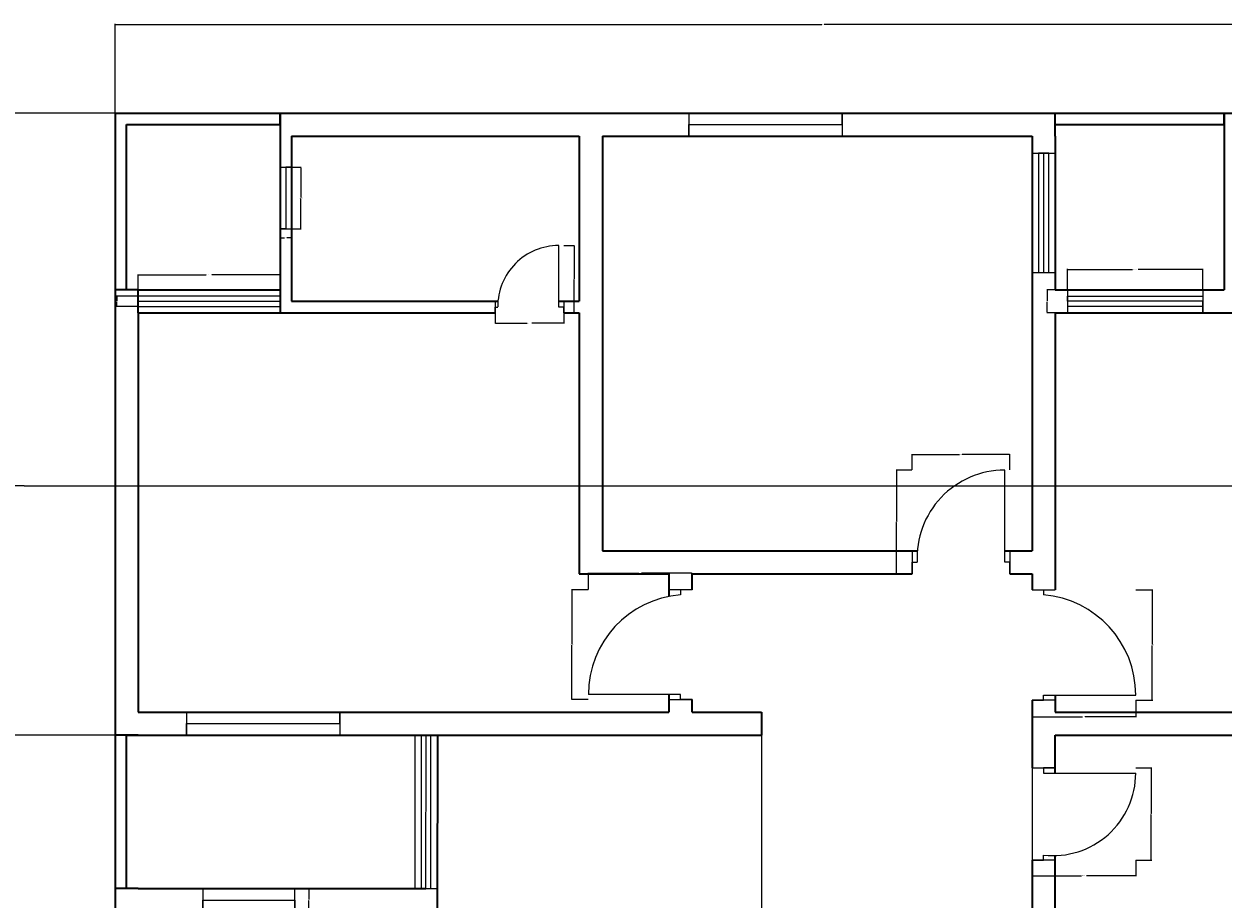
# Model space of a CAD drawing. Units: inches. Extents: x 2014 to 3678, y 870 to 2323.
# Tile 5 of 7: x 2813 to 3282, y 1376 to 1718. Entities that reach past the tile are written whole.
import ezdxf

# ---------------------------------------------------------------- set-up
doc = ezdxf.new("R2010")
doc.units = ezdxf.units.IN
for name, color, linetype, lineweight in [('A-ANNO-DIMS', 2, 'Continuous', 18), ('A-ANNO-SYMB', 2, 'Continuous', 18), ('A-DOOR', 3, 'Continuous', 18), ('A-GLAZ', 4, 'Continuous', 18), ('A-WALL', 7, 'Continuous', 35)]:
    doc.layers.add(name, color=color, linetype=linetype, lineweight=lineweight)
doc.styles.get("Standard").update_dxf_attribs({"font": 'arial.ttf'})
doc.dimstyles.get("Standard").update_dxf_attribs({"dimtxt": 0.18, "dimasz": 0.18, "dimexe": 0.18, "dimexo": 0.0625, "dimgap": 0.09, "dimtad": 0, "dimtih": 1, "dimtoh": 1, "dimdec": 4, "dimzin": 0, "dimdsep": 46, "dimtxsty": 'Standard', "dimcen": 0.09, "dimadec": 0, "dimazin": 0, "dimtfac": 1, "dimtdec": 4, "dimtofl": 0, "dimtmove": 0, "dimatfit": 3, "dimfxl": 1, "dimtolj": 1, "dimtzin": 0, "dimarcsym": 0})

# ---------------------------------------------------------------- blocks, each defined once
blk = doc.blocks.new('DOOR-BATH-WEST-24')
for p, q in [((24.83, 2.25), (24.83, 26.25)), ((0, 4.5), (0, 0)), ((0, 0), (0, 2.25)), ((0, 2.25), (1, 2.25)), ((26.83, 2.25), (24.83, 2.25)), ((26.83, 4.5), (26.83, 0)), ((26.83, 0), (26.83, 2.25))]:
    blk.add_line(p, q)
blk.add_arc((24.83, 2.42), 23.83, 90, 180.4)
blk = doc.blocks.new('DOOR-BED-CENTRE-36')
for p, q in [((36.22, 28.5), (36.22, 40.5)), ((36.22, 4.5), (36.22, 28.5)), ((0, 9), (0, 0)), ((38.22, 9), (38.22, 0)), ((0, 0), (0, 4.5)), ((0, 4.5), (2, 4.5)), ((38.22, 4.5), (36.22, 4.5)), ((38.22, 0), (38.22, 4.5))]:
    blk.add_line(p, q)
blk.add_arc((36.22, 6.23), 34.27, 90, 182.898)
blk = doc.blocks.new('DOOR-BED-WEST-36')
for p, q in [((40.5, 42.9), (31.5, 42.9)), ((36, 42.9), (36, 40.9)), ((36, 2), (0, 2)), ((36, 0), (36, 2)), ((31.5, 0), (40.5, 0)), ((40.5, 0), (36, 0))]:
    blk.add_line(p, q)
blk.add_arc((39.02, 2), 39.02, 94.441, 180)
blk = doc.blocks.new('DOOR-BED-NE-36')
for p, q in [((0, 43.13), (9, 43.13)), ((4.5, 43.13), (4.5, 41.13)), ((9, 0), (0, 0)), ((0, 0), (4.5, 0)), ((4.5, 0), (4.5, 2)), ((4.5, 2), (40.5, 2))]:
    blk.add_line(p, q)
blk.add_arc((1.23, 2), 39.27, 0, 85.2291)
blk = doc.blocks.new('DOOR-BED-SE-36')
for p, q in [((0, 36.03), (9, 36.03)), ((9, 36.03), (4.5, 36.03)), ((4.5, 36.03), (4.5, 34.03)), ((4.5, 34.03), (40.5, 34.03)), ((9, 0), (0, 0)), ((0, 0), (4.5, 0)), ((4.5, 0), (4.5, 2))]:
    blk.add_line(p, q)
blk.add_arc((8.25, 34.03), 32.25, 263.3141, 0)
blk = doc.blocks.new('WIN-60')
for p, q in [((0, 9), (0, 0)), ((60, 4.5), (60, 9)), ((60, 9), (60, 0)), ((0, 0), (0, 4.5)), ((0, 4.5), (60, 4.5))]:
    blk.add_line(p, q)
blk = doc.blocks.new('VENT-24')
for p, q in [((0, 24), (4.5, 24)), ((4.5, 24), (2.25, 24)), ((2.25, 24), (2.25, 0)), ((2.25, 0), (0, 0)), ((0, 0), (4.5, 0))]:
    blk.add_line(p, q)
blk = doc.blocks.new('WIN-36')
for p, q in [((0, 9), (0, 0)), ((36, 0), (36, 9)), ((0, 0), (0, 4.5)), ((0, 4.5), (36, 4.5)), ((36, 4.5), (36, 0))]:
    blk.add_line(p, q)
blk = doc.blocks.new('GLAZ-OTS-EAST')
for p, q in [((0, 9), (0, 0)), ((0, 5.5), (0, 6.5)), ((0, 6.5), (52.91, 6.5)), ((0, 4.5), (0, 5.5)), ((52.91, 9), (52.91, 0)), ((52.91, 6.5), (52.91, 4.5)), ((52.91, 4.5), (0, 4.5)), ((52.91, 2.5), (0, 2.5)), ((52.91, 0), (52.91, 4.5)), ((52.91, 4.5), (52.91, 2.5))]:
    blk.add_line(p, q)
blk = doc.blocks.new('GLAZ-OTS-SIDE')
for p, q in [((0, 46.57), (9, 46.57)), ((4.5, 46.57), (2.5, 46.57)), ((2.5, 46.57), (2.5, 0)), ((4.5, 46.57), (4.5, 0)), ((6.5, 46.57), (4.5, 46.57)), ((6.5, 0), (6.5, 46.57)), ((0, 0), (9, 0)), ((4.5, 0), (6.5, 0))]:
    blk.add_line(p, q)
blk = doc.blocks.new('GLAZ-OTS-WEST')
for p, q in [((55.5, 4), (0, 4)), ((0, 4), (0, 2)), ((0, 2), (55.5, 2)), ((0, 2), (0, 0)), ((0, 0), (55.5, 0)), ((55.5, 2), (55.5, 4))]:
    blk.add_line(p, q)
blk = doc.blocks.new('GLAZ-LAUNDRY')
for p, q in [((9, 60), (0, 60)), ((0, 60), (0, 0)), ((4.5, 60), (2.5, 60)), ((2.5, 60), (2.5, 0)), ((4.35, 0), (4.5, 60)), ((6.35, 0), (6.35, 60)), ((8, 60), (7, 60)), ((9, 60), (8, 60)), ((0, 0), (4.35, 0)), ((2.5, 0), (4.35, 0)), ((4.35, 0), (9, 0.03)), ((7.27, 0.02), (9, 0.03)), ((4.35, 0), (6.35, 0))]:
    blk.add_line(p, q)
blk = doc.blocks.new('*D32')
at = {"layer": 'A-ANNO-DIMS', "color": 0, "lineweight": -2, "transparency": 16777216}
for p, q in [((2917.73, 1662.02), (2921.45, 1662.02)), ((2921.27, 1661.84), (2921.27, 1650.2)), ((2921.27, 1638.2), (2921.27, 1649.84)), ((2917.73, 1638.02), (2921.45, 1638.02))]:
    blk.add_line(p, q, dxfattribs=at)
at = {"layer": 'A-ANNO-DIMS', "color": 0, "transparency": 16777216}
for points in [[(2921.24, 1661.84), (2921.3, 1661.84), (2921.27, 1662.02)], [(2921.24, 1638.2), (2921.3, 1638.2), (2921.27, 1638.02)]]:
    blk.add_solid(points, dxfattribs=at)
at = {"layer": 'Defpoints', "color": 0, "transparency": 16777216}
for p in [(2917.67, 1662.02), (2921.27, 1662.02), (2917.67, 1638.02)]:
    blk.add_point(p, dxfattribs=at)
at = {"layer": 'A-ANNO-DIMS', "color": 0, "transparency": 16777216, "insert": (2921.27, 1650.02), "char_height": 0.18, "attachment_point": 5}
blk.add_mtext('\\A1;VENT 24 TYP.', dxfattribs=at)
blk = doc.blocks.new('*D33')
at = {"layer": 'A-ANNO-DIMS', "color": 0, "lineweight": -2, "transparency": 16777216}
for p, q in [((2913.17, 1637.95), (2913.17, 1634.24)), ((2917.67, 1637.95), (2917.67, 1634.24)), ((2913.35, 1634.42), (2914.96, 1634.42)), ((2917.49, 1634.42), (2915.88, 1634.42))]:
    blk.add_line(p, q, dxfattribs=at)
at = {"layer": 'A-ANNO-DIMS', "color": 0, "transparency": 16777216}
for points in [[(2913.35, 1634.45), (2913.35, 1634.39), (2913.17, 1634.42)], [(2917.49, 1634.45), (2917.49, 1634.39), (2917.67, 1634.42)]]:
    blk.add_solid(points, dxfattribs=at)
at = {"layer": 'Defpoints', "color": 0, "transparency": 16777216}
for p in [(2913.17, 1638.02), (2917.67, 1638.02), (2917.67, 1634.42)]:
    blk.add_point(p, dxfattribs=at)
at = {"layer": 'A-ANNO-DIMS', "color": 0, "transparency": 16777216, "insert": (2915.42, 1634.42), "char_height": 0.18, "attachment_point": 5}
blk.add_mtext('\\A1;5 TYP.', dxfattribs=at)
blk = doc.blocks.new('*D36')
at = {"layer": 'A-ANNO-DIMS', "color": 0, "lineweight": -2, "transparency": 16777216}
for p, q in [((2997.28, 1605.1), (2997.28, 1600.96)), ((3024.11, 1605.1), (3024.11, 1600.96)), ((2997.46, 1601.14), (3009.76, 1601.14)), ((3023.93, 1601.14), (3011.63, 1601.14))]:
    blk.add_line(p, q, dxfattribs=at)
at = {"layer": 'A-ANNO-DIMS', "color": 0, "transparency": 16777216}
for points in [[(2997.46, 1601.17), (2997.46, 1601.11), (2997.28, 1601.14)], [(3023.93, 1601.17), (3023.93, 1601.11), (3024.11, 1601.14)]]:
    blk.add_solid(points, dxfattribs=at)
at = {"layer": 'Defpoints', "color": 0, "transparency": 16777216}
for p in [(2997.28, 1605.17), (3024.11, 1605.17), (3024.11, 1601.14)]:
    blk.add_point(p, dxfattribs=at)
at = {"layer": 'A-ANNO-DIMS', "color": 0, "transparency": 16777216, "insert": (3010.69, 1601.14), "char_height": 0.18, "attachment_point": 5}
blk.add_mtext('\\A1;DOOR 27 TYP.', dxfattribs=at)
blk = doc.blocks.new('*D37')
at = {"layer": 'A-ANNO-DIMS', "color": 0, "lineweight": -2, "transparency": 16777216}
for p, q in [((3024.17, 1631.42), (3028.31, 1631.42)), ((3028.13, 1631.24), (3028.13, 1618.47)), ((3028.13, 1605.35), (3028.13, 1618.11)), ((3024.17, 1605.17), (3028.31, 1605.17))]:
    blk.add_line(p, q, dxfattribs=at)
at = {"layer": 'A-ANNO-DIMS', "color": 0, "transparency": 16777216}
for points in [[(3028.1, 1631.24), (3028.16, 1631.24), (3028.13, 1631.42)], [(3028.1, 1605.35), (3028.16, 1605.35), (3028.13, 1605.17)]]:
    blk.add_solid(points, dxfattribs=at)
at = {"layer": 'Defpoints', "color": 0, "transparency": 16777216}
for p in [(3024.11, 1631.42), (3028.13, 1631.42), (3024.11, 1605.17)]:
    blk.add_point(p, dxfattribs=at)
at = {"layer": 'A-ANNO-DIMS', "color": 0, "transparency": 16777216, "insert": (3028.13, 1618.29), "char_height": 0.18, "attachment_point": 5}
blk.add_mtext('\\A1;26 TYP.', dxfattribs=at)
blk = doc.blocks.new('*D38')
at = {"layer": 'A-ANNO-DIMS', "color": 0, "lineweight": -2, "transparency": 16777216}
for p, q in [((3160.16, 1543.67), (3153.97, 1543.67)), ((3154.15, 1543.49), (3154.15, 1523.6)), ((3154.15, 1503.35), (3154.15, 1523.23)), ((3160.16, 1503.17), (3153.97, 1503.17))]:
    blk.add_line(p, q, dxfattribs=at)
at = {"layer": 'A-ANNO-DIMS', "color": 0, "transparency": 16777216}
for points in [[(3154.12, 1543.49), (3154.18, 1543.49), (3154.15, 1543.67)], [(3154.12, 1503.35), (3154.18, 1503.35), (3154.15, 1503.17)]]:
    blk.add_solid(points, dxfattribs=at)
at = {"layer": 'Defpoints', "color": 0, "transparency": 16777216}
for p in [(3154.15, 1543.67), (3160.23, 1543.67), (3160.23, 1503.17)]:
    blk.add_point(p, dxfattribs=at)
at = {"layer": 'A-ANNO-DIMS', "color": 0, "transparency": 16777216, "insert": (3154.15, 1523.42), "char_height": 0.18, "attachment_point": 5}
blk.add_mtext('\\A1;DOOR 41 TYP.', dxfattribs=at)
blk = doc.blocks.new('*D39')
at = {"layer": 'A-ANNO-DIMS', "color": 0, "lineweight": -2, "transparency": 16777216}
for p, q in [((3160.23, 1543.73), (3160.23, 1549.92)), ((3160.41, 1549.74), (3178.81, 1549.74)), ((3198.27, 1549.74), (3179.87, 1549.74)), ((3198.45, 1543.73), (3198.45, 1549.92))]:
    blk.add_line(p, q, dxfattribs=at)
at = {"layer": 'A-ANNO-DIMS', "color": 0, "transparency": 16777216}
for points in [[(3160.41, 1549.77), (3160.41, 1549.71), (3160.23, 1549.74)], [(3198.27, 1549.77), (3198.27, 1549.71), (3198.45, 1549.74)]]:
    blk.add_solid(points, dxfattribs=at)
at = {"layer": 'Defpoints', "color": 0, "transparency": 16777216}
for p in [(3198.45, 1549.74), (3160.23, 1543.67), (3198.45, 1543.67)]:
    blk.add_point(p, dxfattribs=at)
at = {"layer": 'A-ANNO-DIMS', "color": 0, "transparency": 16777216, "insert": (3179.34, 1549.74), "char_height": 0.18, "attachment_point": 5}
blk.add_mtext('\\A1;38 TYP.', dxfattribs=at)
blk = doc.blocks.new('*D40')
at = {"layer": 'A-ANNO-DIMS', "color": 0, "lineweight": -2, "transparency": 16777216}
for p, q in [((3033.65, 1496.94), (3027.1, 1496.94)), ((3027.28, 1496.76), (3027.28, 1475.67)), ((3027.28, 1454.21), (3027.28, 1475.3)), ((3033.65, 1454.03), (3027.1, 1454.03))]:
    blk.add_line(p, q, dxfattribs=at)
at = {"layer": 'A-ANNO-DIMS', "color": 0, "transparency": 16777216}
for points in [[(3027.25, 1496.76), (3027.31, 1496.76), (3027.28, 1496.94)], [(3027.25, 1454.21), (3027.31, 1454.21), (3027.28, 1454.03)]]:
    blk.add_solid(points, dxfattribs=at)
at = {"layer": 'Defpoints', "color": 0, "transparency": 16777216}
for p in [(3027.28, 1496.94), (3033.71, 1496.94), (3033.71, 1454.03)]:
    blk.add_point(p, dxfattribs=at)
at = {"layer": 'A-ANNO-DIMS', "color": 0, "transparency": 16777216, "insert": (3027.28, 1475.49), "char_height": 0.18, "attachment_point": 5}
blk.add_mtext('\\A1;DOOR 43 TYP.', dxfattribs=at)
blk = doc.blocks.new('*D41')
at = {"layer": 'A-ANNO-DIMS', "color": 0, "lineweight": -2, "transparency": 16777216}
for p, q in [((3033.71, 1497), (3033.71, 1503.55)), ((3033.89, 1503.37), (3053.43, 1503.37)), ((3074.03, 1503.37), (3054.5, 1503.37)), ((3074.21, 1497), (3074.21, 1503.55))]:
    blk.add_line(p, q, dxfattribs=at)
at = {"layer": 'A-ANNO-DIMS', "color": 0, "transparency": 16777216}
for points in [[(3033.89, 1503.4), (3033.89, 1503.34), (3033.71, 1503.37)], [(3074.03, 1503.4), (3074.03, 1503.34), (3074.21, 1503.37)]]:
    blk.add_solid(points, dxfattribs=at)
at = {"layer": 'Defpoints', "color": 0, "transparency": 16777216}
for p in [(3074.21, 1503.37), (3033.71, 1496.94), (3074.21, 1496.94)]:
    blk.add_point(p, dxfattribs=at)
at = {"layer": 'A-ANNO-DIMS', "color": 0, "transparency": 16777216, "insert": (3053.96, 1503.37), "char_height": 0.18, "attachment_point": 5}
blk.add_mtext('\\A1;41 TYP.', dxfattribs=at)
blk = doc.blocks.new('*D42')
at = {"layer": 'A-ANNO-DIMS', "color": 0, "lineweight": -2, "transparency": 16777216}
for p, q in [((3247.73, 1496.94), (3254.32, 1496.94)), ((3254.14, 1496.76), (3254.14, 1475.56)), ((3254.14, 1453.99), (3254.14, 1475.19)), ((3247.73, 1453.81), (3254.32, 1453.81))]:
    blk.add_line(p, q, dxfattribs=at)
at = {"layer": 'A-ANNO-DIMS', "color": 0, "transparency": 16777216}
for points in [[(3254.11, 1496.76), (3254.17, 1496.76), (3254.14, 1496.94)], [(3254.11, 1453.99), (3254.17, 1453.99), (3254.14, 1453.81)]]:
    blk.add_solid(points, dxfattribs=at)
at = {"layer": 'Defpoints', "color": 0, "transparency": 16777216}
for p in [(3247.67, 1496.94), (3254.14, 1496.94), (3247.67, 1453.81)]:
    blk.add_point(p, dxfattribs=at)
at = {"layer": 'A-ANNO-DIMS', "color": 0, "transparency": 16777216, "insert": (3254.14, 1475.37), "char_height": 0.18, "attachment_point": 5}
blk.add_mtext('\\A1;DOOR 43 TYP.', dxfattribs=at)
blk = doc.blocks.new('*D43')
at = {"layer": 'A-ANNO-DIMS', "color": 0, "lineweight": -2, "transparency": 16777216}
for p, q in [((3207.17, 1453.75), (3207.17, 1447.16)), ((3247.67, 1453.75), (3247.67, 1447.16)), ((3207.35, 1447.34), (3226.89, 1447.34)), ((3247.49, 1447.34), (3227.95, 1447.34))]:
    blk.add_line(p, q, dxfattribs=at)
at = {"layer": 'A-ANNO-DIMS', "color": 0, "transparency": 16777216}
for points in [[(3207.35, 1447.37), (3207.35, 1447.31), (3207.17, 1447.34)], [(3247.49, 1447.37), (3247.49, 1447.31), (3247.67, 1447.34)]]:
    blk.add_solid(points, dxfattribs=at)
at = {"layer": 'Defpoints', "color": 0, "transparency": 16777216}
for p in [(3207.17, 1453.81), (3247.67, 1453.81), (3247.67, 1447.34)]:
    blk.add_point(p, dxfattribs=at)
at = {"layer": 'A-ANNO-DIMS', "color": 0, "transparency": 16777216, "insert": (3227.42, 1447.34), "char_height": 0.18, "attachment_point": 5}
blk.add_mtext('\\A1;41 TYP.', dxfattribs=at)
blk = doc.blocks.new('*D44')
at = {"layer": 'A-ANNO-DIMS', "color": 0, "lineweight": -2, "transparency": 16777216}
for p, q in [((3207.17, 1391.22), (3207.17, 1385.03)), ((3247.67, 1391.22), (3247.67, 1385.03)), ((3207.35, 1385.21), (3226.49, 1385.21)), ((3247.49, 1385.21), (3228.36, 1385.21))]:
    blk.add_line(p, q, dxfattribs=at)
at = {"layer": 'A-ANNO-DIMS', "color": 0, "transparency": 16777216}
for points in [[(3207.35, 1385.24), (3207.35, 1385.18), (3207.17, 1385.21)], [(3247.49, 1385.24), (3247.49, 1385.18), (3247.67, 1385.21)]]:
    blk.add_solid(points, dxfattribs=at)
at = {"layer": 'Defpoints', "color": 0, "transparency": 16777216}
for p in [(3207.17, 1391.28), (3247.67, 1391.28), (3247.67, 1385.21)]:
    blk.add_point(p, dxfattribs=at)
at = {"layer": 'A-ANNO-DIMS', "color": 0, "transparency": 16777216, "insert": (3227.42, 1385.21), "char_height": 0.18, "attachment_point": 5}
blk.add_mtext('\\A1;DOOR 41 TYP.', dxfattribs=at)
blk = doc.blocks.new('*D45')
at = {"layer": 'A-ANNO-DIMS', "color": 0, "lineweight": -2, "transparency": 16777216}
for p, q in [((3247.73, 1427.31), (3253.93, 1427.31)), ((3253.75, 1427.13), (3253.75, 1409.48)), ((3253.75, 1391.46), (3253.75, 1409.11)), ((3247.73, 1391.28), (3253.93, 1391.28))]:
    blk.add_line(p, q, dxfattribs=at)
at = {"layer": 'A-ANNO-DIMS', "color": 0, "transparency": 16777216}
for points in [[(3253.72, 1427.13), (3253.78, 1427.13), (3253.75, 1427.31)], [(3253.72, 1391.46), (3253.78, 1391.46), (3253.75, 1391.28)]]:
    blk.add_solid(points, dxfattribs=at)
at = {"layer": 'Defpoints', "color": 0, "transparency": 16777216}
for p in [(3247.67, 1427.31), (3253.75, 1427.31), (3247.67, 1391.28)]:
    blk.add_point(p, dxfattribs=at)
at = {"layer": 'A-ANNO-DIMS', "color": 0, "transparency": 16777216, "insert": (3253.75, 1409.29), "char_height": 0.18, "attachment_point": 5}
blk.add_mtext('\\A1;36 TYP.', dxfattribs=at)
blk = doc.blocks.new('*D55')
at = {"layer": 'A-ANNO-DIMS', "color": 0, "lineweight": -2, "transparency": 16777216}
for p, q in [((2919.09, 1380.17), (2924.6, 1380.17)), ((2924.42, 1379.99), (2924.42, 1375.85)), ((2924.42, 1371.35), (2924.42, 1375.48)), ((2919.09, 1371.17), (2924.6, 1371.17))]:
    blk.add_line(p, q, dxfattribs=at)
at = {"layer": 'A-ANNO-DIMS', "color": 0, "transparency": 16777216}
for points in [[(2924.39, 1379.99), (2924.45, 1379.99), (2924.42, 1380.17)], [(2924.39, 1371.35), (2924.45, 1371.35), (2924.42, 1371.17)]]:
    blk.add_solid(points, dxfattribs=at)
at = {"layer": 'Defpoints', "color": 0, "transparency": 16777216}
for p in [(2919.02, 1380.17), (2924.42, 1380.17), (2919.02, 1371.17)]:
    blk.add_point(p, dxfattribs=at)
at = {"layer": 'A-ANNO-DIMS', "color": 0, "transparency": 16777216, "insert": (2924.42, 1375.67), "char_height": 0.18, "attachment_point": 5}
blk.add_mtext('\\A1;9 TYP.', dxfattribs=at)
blk = doc.blocks.new('*D56')
at = {"layer": 'A-ANNO-DIMS', "color": 0, "lineweight": -2, "transparency": 16777216}
for p, q in [((3221.02, 1614.23), (3221.02, 1622.28)), ((3221.2, 1622.1), (3246.36, 1622.1)), ((3273.75, 1622.1), (3248.59, 1622.1)), ((3273.93, 1614.23), (3273.93, 1622.28))]:
    blk.add_line(p, q, dxfattribs=at)
at = {"layer": 'A-ANNO-DIMS', "color": 0, "transparency": 16777216}
for points in [[(3221.2, 1622.13), (3221.2, 1622.07), (3221.02, 1622.1)], [(3273.75, 1622.13), (3273.75, 1622.07), (3273.93, 1622.1)]]:
    blk.add_solid(points, dxfattribs=at)
at = {"layer": 'Defpoints', "color": 0, "transparency": 16777216}
for p in [(3273.93, 1622.1), (3221.02, 1614.17), (3273.93, 1614.17)]:
    blk.add_point(p, dxfattribs=at)
at = {"layer": 'A-ANNO-DIMS', "color": 0, "transparency": 16777216, "insert": (3247.48, 1622.1), "char_height": 0.18, "attachment_point": 5}
blk.add_mtext('\\A1;GLAZING 53 TYP.', dxfattribs=at)
blk = doc.blocks.new('*D57')
at = {"layer": 'A-ANNO-DIMS', "color": 0, "lineweight": -2, "transparency": 16777216}
for p, q in [((3220.96, 1614.17), (3212.91, 1614.17)), ((3213.09, 1613.99), (3213.09, 1609.85)), ((3213.09, 1605.35), (3213.09, 1609.48)), ((3220.96, 1605.17), (3212.91, 1605.17))]:
    blk.add_line(p, q, dxfattribs=at)
at = {"layer": 'A-ANNO-DIMS', "color": 0, "transparency": 16777216}
for points in [[(3213.06, 1613.99), (3213.12, 1613.99), (3213.09, 1614.17)], [(3213.06, 1605.35), (3213.12, 1605.35), (3213.09, 1605.17)]]:
    blk.add_solid(points, dxfattribs=at)
at = {"layer": 'Defpoints', "color": 0, "transparency": 16777216}
for p in [(3213.09, 1614.17), (3221.02, 1614.17), (3221.02, 1605.17)]:
    blk.add_point(p, dxfattribs=at)
at = {"layer": 'A-ANNO-DIMS', "color": 0, "transparency": 16777216, "insert": (3213.09, 1609.67), "char_height": 0.18, "attachment_point": 5}
blk.add_mtext('\\A1;9 TYP.', dxfattribs=at)
blk = doc.blocks.new('*D60')
at = {"layer": 'A-ANNO-DIMS', "color": 0, "lineweight": -2, "transparency": 16777216}
for p, q in [((2857.67, 1611.73), (2857.67, 1620.17)), ((2857.85, 1619.99), (2884.31, 1619.99)), ((2912.99, 1619.99), (2886.54, 1619.99)), ((2913.17, 1611.73), (2913.17, 1620.17))]:
    blk.add_line(p, q, dxfattribs=at)
at = {"layer": 'A-ANNO-DIMS', "color": 0, "transparency": 16777216}
for points in [[(2857.85, 1620.02), (2857.85, 1619.96), (2857.67, 1619.99)], [(2912.99, 1620.02), (2912.99, 1619.96), (2913.17, 1619.99)]]:
    blk.add_solid(points, dxfattribs=at)
at = {"layer": 'Defpoints', "color": 0, "transparency": 16777216}
for p in [(2913.17, 1619.99), (2857.67, 1611.67), (2913.17, 1611.67)]:
    blk.add_point(p, dxfattribs=at)
at = {"layer": 'A-ANNO-DIMS', "color": 0, "transparency": 16777216, "insert": (2885.42, 1619.99), "char_height": 0.18, "attachment_point": 5}
blk.add_mtext('\\A1;GLAZING 56 TYP.', dxfattribs=at)
blk = doc.blocks.new('*D61')
at = {"layer": 'A-ANNO-DIMS', "color": 0, "lineweight": -2, "transparency": 16777216}
for p, q in [((2857.61, 1611.67), (2849.17, 1611.67)), ((2849.35, 1611.49), (2849.35, 1609.85)), ((2849.35, 1607.85), (2849.35, 1609.49)), ((2857.61, 1607.67), (2849.17, 1607.67))]:
    blk.add_line(p, q, dxfattribs=at)
at = {"layer": 'A-ANNO-DIMS', "color": 0, "transparency": 16777216}
for points in [[(2849.32, 1611.49), (2849.38, 1611.49), (2849.35, 1611.67)], [(2849.32, 1607.85), (2849.38, 1607.85), (2849.35, 1607.67)]]:
    blk.add_solid(points, dxfattribs=at)
at = {"layer": 'Defpoints', "color": 0, "transparency": 16777216}
for p in [(2849.35, 1611.67), (2857.67, 1611.67), (2857.67, 1607.67)]:
    blk.add_point(p, dxfattribs=at)
at = {"layer": 'A-ANNO-DIMS', "color": 0, "transparency": 16777216, "insert": (2849.35, 1609.67), "char_height": 0.18, "attachment_point": 5}
blk.add_mtext('\\A1;4 TYP.', dxfattribs=at)
blk = doc.blocks.new('*D91')
at = {"layer": 'A-ANNO-DIMS', "color": 0, "lineweight": -2, "transparency": 16777216}
for p, q in [((2848.67, 1683.23), (2848.67, 1718)), ((2848.85, 1717.82), (3125.03, 1717.82)), ((3401.99, 1717.82), (3125.82, 1717.82)), ((3402.17, 1683.23), (3402.17, 1718))]:
    blk.add_line(p, q, dxfattribs=at)
at = {"layer": 'A-ANNO-DIMS', "color": 0, "transparency": 16777216}
for points in [[(2848.85, 1717.85), (2848.85, 1717.79), (2848.67, 1717.82)], [(3401.99, 1717.85), (3401.99, 1717.79), (3402.17, 1717.82)]]:
    blk.add_solid(points, dxfattribs=at)
at = {"layer": 'Defpoints', "color": 0, "transparency": 16777216}
for p in [(3402.17, 1717.82), (2848.67, 1683.17), (3402.17, 1683.17)]:
    blk.add_point(p, dxfattribs=at)
at = {"layer": 'A-ANNO-DIMS', "color": 0, "transparency": 16777216, "insert": (3125.42, 1717.82), "char_height": 0.18, "attachment_point": 5}
blk.add_mtext('\\A1;553.5', dxfattribs=at)
blk = doc.blocks.new('*D95')
at = {"layer": 'A-ANNO-DIMS', "color": 0, "lineweight": -2, "transparency": 16777216}
for p, q in [((2848.61, 1440.17), (2778.34, 1440.17)), ((2778.52, 1439.99), (2778.52, 1405.85)), ((2778.52, 1371.35), (2778.52, 1405.48)), ((2857.61, 1371.17), (2778.34, 1371.17))]:
    blk.add_line(p, q, dxfattribs=at)
at = {"layer": 'A-ANNO-DIMS', "color": 0, "transparency": 16777216}
for points in [[(2778.49, 1439.99), (2778.55, 1439.99), (2778.52, 1440.17)], [(2778.49, 1371.35), (2778.55, 1371.35), (2778.52, 1371.17)]]:
    blk.add_solid(points, dxfattribs=at)
at = {"layer": 'Defpoints', "color": 0, "transparency": 16777216}
for p in [(2778.52, 1440.17), (2848.67, 1440.17), (2857.67, 1371.17)]:
    blk.add_point(p, dxfattribs=at)
at = {"layer": 'A-ANNO-DIMS', "color": 0, "transparency": 16777216, "insert": (2778.52, 1405.67), "char_height": 0.18, "attachment_point": 5}
blk.add_mtext('\\A1;69', dxfattribs=at)
blk = doc.blocks.new('*D96')
at = {"layer": 'A-ANNO-DIMS', "color": 0, "lineweight": -2, "transparency": 16777216}
for p, q in [((2813.11, 1537.5), (2778.34, 1537.5)), ((2778.52, 1537.32), (2778.52, 1489.01)), ((2778.52, 1440.35), (2778.52, 1488.65)), ((2848.61, 1440.17), (2778.34, 1440.17))]:
    blk.add_line(p, q, dxfattribs=at)
at = {"layer": 'A-ANNO-DIMS', "color": 0, "transparency": 16777216}
for points in [[(2778.49, 1537.32), (2778.55, 1537.32), (2778.52, 1537.5)], [(2778.49, 1440.35), (2778.55, 1440.35), (2778.52, 1440.17)]]:
    blk.add_solid(points, dxfattribs=at)
at = {"layer": 'Defpoints', "color": 0, "transparency": 16777216}
for p in [(2778.52, 1537.5), (2813.17, 1537.5), (2848.67, 1440.17)]:
    blk.add_point(p, dxfattribs=at)
at = {"layer": 'A-ANNO-DIMS', "color": 0, "transparency": 16777216, "insert": (2778.52, 1488.83), "char_height": 0.18, "attachment_point": 5}
blk.add_mtext('\\A1;97.33', dxfattribs=at)
blk = doc.blocks.new('*D97')
at = {"layer": 'A-ANNO-DIMS', "color": 0, "lineweight": -2, "transparency": 16777216}
for p, q in [((2848.61, 1683.17), (2778.34, 1683.17)), ((2778.52, 1682.99), (2778.52, 1610.51)), ((2778.52, 1537.68), (2778.52, 1610.15)), ((2813.11, 1537.5), (2778.34, 1537.5))]:
    blk.add_line(p, q, dxfattribs=at)
at = {"layer": 'A-ANNO-DIMS', "color": 0, "transparency": 16777216}
for points in [[(2778.49, 1682.99), (2778.55, 1682.99), (2778.52, 1683.17)], [(2778.49, 1537.68), (2778.55, 1537.68), (2778.52, 1537.5)]]:
    blk.add_solid(points, dxfattribs=at)
at = {"layer": 'Defpoints', "color": 0, "transparency": 16777216}
for p in [(2778.52, 1683.17), (2848.67, 1683.17), (2813.17, 1537.5)]:
    blk.add_point(p, dxfattribs=at)
at = {"layer": 'A-ANNO-DIMS', "color": 0, "transparency": 16777216, "insert": (2778.52, 1610.33), "char_height": 0.18, "attachment_point": 5}
blk.add_mtext('\\A1;145.67', dxfattribs=at)
blk = doc.blocks.new('*D100')
at = {"layer": 'A-ANNO-DIMS', "color": 0, "lineweight": -2, "transparency": 16777216}
for p, q in [((3101.37, 1440.1), (3101.37, 964.34)), ((3207.17, 1427.25), (3207.17, 964.34)), ((3101.55, 964.52), (3153.88, 964.52)), ((3206.99, 964.52), (3154.65, 964.52))]:
    blk.add_line(p, q, dxfattribs=at)
at = {"layer": 'A-ANNO-DIMS', "color": 0, "transparency": 16777216}
for points in [[(3101.55, 964.55), (3101.55, 964.49), (3101.37, 964.52)], [(3206.99, 964.55), (3206.99, 964.49), (3207.17, 964.52)]]:
    blk.add_solid(points, dxfattribs=at)
at = {"layer": 'Defpoints', "color": 0, "transparency": 16777216}
for p in [(3101.37, 1440.17), (3207.17, 1427.31), (3207.17, 964.52)]:
    blk.add_point(p, dxfattribs=at)
at = {"layer": 'A-ANNO-DIMS', "color": 0, "transparency": 16777216, "insert": (3154.27, 964.52), "char_height": 0.18, "attachment_point": 5}
blk.add_mtext('\\A1;105.8', dxfattribs=at)

msp = doc.modelspace()

# ---------------------------------------------------------------- linework, layer by layer
at = {"layer": 'A-ANNO-SYMB'}
msp.add_line((2813.1731, 1537.5002), (3449.5026, 1537.5002), dxfattribs=at)
at = {"layer": 'A-WALL'}
for p, q in [((2848.6718, 1683.1655), (3402.1718, 1683.1655)), ((2848.6718, 1683.1655), (3402.1718, 1683.1655)), ((2848.6718, 1683.1655), (2848.6718, 1083.1655)), ((2913.1718, 1678.6655), (2913.1718, 1683.1655)), ((2913.1718, 1683.1655), (2913.1718, 1674.1655)), ((3216.1718, 1678.6655), (3216.1718, 1683.1655)), ((3282.1718, 1678.6655), (3282.1718, 1683.1655)), ((3282.1718, 1683.1655), (3282.1718, 1674.1655)), ((2853.1718, 1614.1655), (2853.1718, 1678.6655)), ((2853.1718, 1678.6655), (2913.1718, 1678.6655)), ((3216.1718, 1674.1655), (3216.1718, 1678.6655)), ((3216.1718, 1678.6655), (3282.1718, 1678.6655)), ((2913.1718, 1674.1655), (2913.1718, 1605.1655)), ((2917.6718, 1674.1655), (3030.1718, 1674.1655)), ((2917.6718, 1674.1655), (2917.6718, 1614.1655)), ((3030.1718, 1674.1655), (3030.1718, 1609.6655)), ((3039.1718, 1674.1655), (3207.1718, 1674.1655)), ((3039.1718, 1674.1655), (3039.1718, 1512.1655)), ((3207.1718, 1674.1655), (3207.1718, 1614.1655)), ((3216.1718, 1674.1655), (3216.1718, 1614.1655)), ((3282.1718, 1674.1655), (3282.1718, 1614.1655)), ((3207.1718, 1620.9201), (3207.1718, 1512.1655)), ((2857.6718, 1614.1655), (2848.6718, 1614.1655)), ((2857.6718, 1614.1655), (2853.1718, 1614.1655)), ((2857.6718, 1614.1655), (2913.1718, 1614.1655)), ((2857.6718, 1605.1655), (2857.6718, 1614.1655)), ((2917.6718, 1614.1655), (2917.6718, 1609.6655)), ((3216.1718, 1614.1655), (3282.1718, 1614.1655)), ((2917.6718, 1609.6655), (2998.3665, 1609.6655)), ((3022.1088, 1609.6655), (3030.1718, 1609.6655)), ((2857.6718, 1605.1655), (2997.2758, 1605.1655)), ((2857.6718, 1605.1655), (2857.6718, 1449.1655)), ((3024.1088, 1605.1655), (3030.1718, 1605.1655)), ((3030.1718, 1605.1655), (3030.1718, 1503.1655)), ((3216.1718, 1605.1655), (3360.6647, 1605.1655)), ((3216.1718, 1605.1655), (3216.1718, 1503.1655)), ((3039.1718, 1512.1655), (3162.2942, 1512.1655)), ((3196.4497, 1512.1655), (3207.1718, 1512.1655)), ((3030.1718, 1503.1655), (3065.2147, 1503.1655)), ((3065.2147, 1503.1655), (3065.2147, 1494.3233)), ((3074.2147, 1503.1655), (3160.2261, 1503.1655)), ((3074.2147, 1496.9379), (3074.2147, 1503.1655)), ((3198.4497, 1503.1655), (3207.1718, 1503.1655)), ((3207.1718, 1503.1655), (3207.1718, 1496.9379)), ((3216.1718, 1503.1655), (3216.1718, 1496.9379)), ((3065.2147, 1456.0336), (3065.2147, 1449.1655)), ((3216.1718, 1455.8082), (3216.1718, 1449.1655)), ((3074.2147, 1449.1655), (3074.2147, 1454.0336)), ((3207.1718, 1453.8082), (3207.1718, 1440.1655)), ((2857.6718, 1449.1655), (3065.2147, 1449.1655)), ((2970.1718, 1449.1655), (2979.1718, 1449.1655)), ((3074.2147, 1449.1655), (3101.3665, 1449.1655)), ((3101.3665, 1449.1655), (3101.3665, 1440.1655)), ((3216.1718, 1449.1655), (3393.1718, 1449.1655)), ((2857.6718, 1440.1655), (2848.6718, 1440.1655)), ((2853.1718, 1380.1655), (2853.1718, 1440.1655)), ((2853.1718, 1440.1655), (2857.6718, 1440.1655)), ((2857.6718, 1440.1655), (2970.1718, 1440.1655)), ((2970.1718, 1440.1655), (2979.2119, 1440.1655)), ((2974.6718, 1371.1655), (2974.8253, 1440.1655)), ((2979.2119, 1440.1655), (3101.3665, 1440.1655)), ((3207.1718, 1440.1655), (3207.1718, 1427.3075)), ((3216.1718, 1440.1655), (3393.1718, 1440.1655)), ((3216.1718, 1425.3075), (3216.1718, 1440.1655)), ((3207.1718, 1391.2811), (3207.1718, 1275.1655)), ((3216.1718, 1284.1655), (3216.1718, 1393.0704)), ((2853.1718, 1380.1655), (2848.6718, 1380.1655)), ((2857.6718, 1380.1655), (2853.1718, 1380.1655)), ((2857.6718, 1380.1655), (2970.1718, 1380.1655))]:
    msp.add_line(p, q, dxfattribs=at)

# ---------------------------------------------------------------- block references
at = {"layer": 'A-DOOR'}
for name, p in [('DOOR-BATH-WEST-24', (2997.2761, 1605.165)), ('DOOR-BED-CENTRE-36', (3160.2261, 1503.165)), ('DOOR-BED-WEST-36', (3033.7151, 1454.034)), ('DOOR-BED-NE-36', (3207.1721, 1453.808)), ('DOOR-BED-SE-36', (3207.1721, 1391.281))]:
    msp.add_blockref(name, p, dxfattribs=at)
at = {"layer": 'A-GLAZ'}
for name, p in [('WIN-60', (3072.9262, 1674.165)), ('GLAZ-OTS-SIDE', (3207.1721, 1620.92)), ('VENT-24', (2913.1721, 1638.0168)), ('GLAZ-OTS-EAST', (3221.0211, 1605.165)), ('GLAZ-OTS-WEST', (2857.6721, 1607.665)), ('WIN-60', (2876.5803, 1440.165)), ('GLAZ-LAUNDRY', (2965.8251, 1380.161)), ('WIN-36', (2883.0251, 1371.165))]:
    msp.add_blockref(name, p, dxfattribs=at)

# ---------------------------------------------------------------- dimensions: what is measured, and where the dimension line sits
at = {"layer": 'A-ANNO-DIMS'}
for base, p1, p2, picture, middle in [((3402.1718, 1717.8155), (2848.6718, 1683.1655), (3402.1718, 1683.1655), '*D91', (3125.4218, 1717.8155)), ((3207.1718, 964.5155), (3101.3665, 1440.1655), (3207.1718, 1427.3075), '*D100', (3154.2691, 964.5155))]:
    dim = msp.add_linear_dim(base=base, p1=p1, p2=p2, dimstyle='Standard', override={"dimdec": 1, "dimlfac": 1, "dimrnd": 0, "dimzin": 0, "dimdsep": 46, "dimlunit": 2}, dxfattribs=at)
    dim.commit()
    dim.dimension.update_dxf_attribs({"geometry": picture, "text_midpoint": middle})
for base, p1, p2, override, picture, middle in [((2778.5231, 1683.1655), (2813.1731, 1537.5002), (2848.6718, 1683.1655), {"dimdec": 2, "dimlfac": 1, "dimrnd": 0, "dimzin": 0, "dimdsep": 46, "dimlunit": 2}, '*D97', (2778.5231, 1610.3328)), ((2778.5231, 1537.5002), (2848.6718, 1440.1655), (2813.1731, 1537.5002), {"dimdec": 2, "dimlfac": 1, "dimrnd": 0, "dimzin": 0, "dimdsep": 46, "dimlunit": 2}, '*D96', (2778.5231, 1488.8328)), ((2778.5231, 1440.1655), (2857.6718, 1371.1655), (2848.6718, 1440.1655), {"dimdec": 0, "dimlfac": 1, "dimrnd": 0, "dimzin": 0, "dimdsep": 46, "dimlunit": 2}, '*D95', (2778.5231, 1405.6655))]:
    dim = msp.add_linear_dim(base=base, p1=p1, p2=p2, angle=90, dimstyle='Standard', override=override, dxfattribs=at)
    dim.commit()
    dim.dimension.update_dxf_attribs({"geometry": picture, "text_midpoint": middle})
for base, p1, p2, text, picture, middle in [((2921.2718, 1662.0164), (2917.6718, 1638.0164), (2917.6718, 1662.0164), 'VENT <> TYP.', '*D32', (2921.2718, 1650.0164)), ((3028.1338, 1631.4155), (3024.1088, 1605.1655), (3024.1088, 1631.4155), '<> TYP.', '*D37', (3028.1338, 1618.2905)), ((3213.0854, 1614.1655), (3221.0216, 1605.1655), (3221.0216, 1614.1655), '<> TYP.', '*D57', (3213.0854, 1609.6655)), ((2849.3468, 1611.6655), (2857.6718, 1607.6655), (2857.6718, 1611.6655), '<> TYP.', '*D61', (2849.3468, 1609.6655)), ((3154.1510618452, 1543.6654745472), (3160.2260618452, 1503.1654745472), (3160.2260618452, 1543.6654745472), 'DOOR <> TYP.', '*D38', (3154.1510618452, 1523.4154745472)), ((3027.279, 1496.9379), (3033.7147, 1454.0336), (3033.7147, 1496.9379), 'DOOR <> TYP.', '*D40', (3027.279, 1475.4858)), ((3254.1413, 1496.9379), (3247.6718, 1453.8082), (3247.6718, 1496.9379), 'DOOR <> TYP.', '*D42', (3254.1413, 1475.3731)), ((3253.7468, 1427.3075), (3247.6718, 1391.2811), (3247.6718, 1427.3075), '<> TYP.', '*D45', (3253.7468, 1409.2943)), ((2924.4246, 1380.1655), (2919.0246, 1371.1655), (2919.0246, 1380.1655), '<> TYP.', '*D55', (2924.4246, 1375.6655))]:
    dim = msp.add_linear_dim(base=base, p1=p1, p2=p2, angle=90, text=text, dimstyle='Standard', override={"dimdec": 0, "dimlfac": 1, "dimrnd": 0, "dimzin": 0, "dimdsep": 46, "dimlunit": 2}, dxfattribs=at)
    dim.commit()
    dim.dimension.update_dxf_attribs({"geometry": picture, "text_midpoint": middle})
for base, p1, p2, text, picture, middle in [((2917.6717955133, 1634.4163578635), (2913.1717955133, 1638.0163578635), (2917.6717955133, 1638.0163578635), '<> TYP.', '*D33', (2915.4217955133, 1634.4163578635)), ((2913.1717955133, 1619.9904745472), (2857.6717955133, 1611.6654745472), (2913.1717955133, 1611.6654745472), 'GLAZING <> TYP.', '*D60', (2885.4217955133, 1619.9904745472)), ((3273.9293, 1622.1016), (3221.0216, 1614.1655), (3273.9293, 1614.1655), 'GLAZING <> TYP.', '*D56', (3247.4754, 1622.1016)), ((3024.1088, 1601.1405), (2997.2758, 1605.1655), (3024.1088, 1605.1655), 'DOOR <> TYP.', '*D36', (3010.6923, 1601.1405)), ((3198.4497, 1549.7405), (3160.2261, 1543.6655), (3198.4497, 1543.6655), '<> TYP.', '*D39', (3179.3379, 1549.7405)), ((3074.2147013089, 1503.3735923131), (3033.7147013089, 1496.9379382809), (3074.2147013089, 1496.9379382809), '<> TYP.', '*D41', (3053.9647013089, 1503.3735923131)), ((3247.6717955133, 1447.3387139967), (3207.1717955133, 1453.8081780338), (3247.6717955133, 1453.8081780338), '<> TYP.', '*D43', (3227.4217955133, 1447.3387139967)), ((3247.6717955133, 1385.2060872063), (3207.1717955133, 1391.2810872063), (3247.6717955133, 1391.2810872063), 'DOOR <> TYP.', '*D44', (3227.4217955133, 1385.2060872063))]:
    dim = msp.add_linear_dim(base=base, p1=p1, p2=p2, text=text, dimstyle='Standard', override={"dimdec": 0, "dimlfac": 1, "dimrnd": 0, "dimzin": 0, "dimdsep": 46, "dimlunit": 2}, dxfattribs=at)
    dim.commit()
    dim.dimension.update_dxf_attribs({"geometry": picture, "text_midpoint": middle})

doc.saveas('drawing.dxf')
